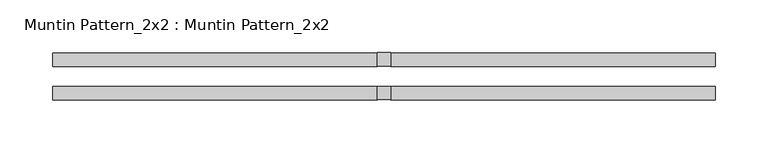
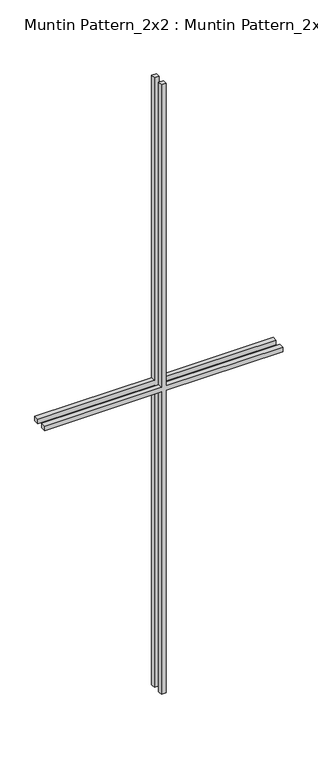
"""IFC4 building model written with IfcOpenShell, lengths in millimetres: proxy geometry, Muntin Pattern_2x2 : Muntin Pattern_2x2."""

from ifc_helpers import new_model, si_unit, frame, origin, place, context, project, spatial, polyline, outline, extrude, source, transform, mapped, element, save


def muntin_pattern_2x2_muntin_pattern_2x2_09b00a1c(model_context):
    return source(origin(), model_context, "Body", "SweptSolid", [
        extrude(outline(polyline([(850.9, -6.35), (850.9, -312.7375), (838.2, -312.7375), (838.2, -6.35), (0.0, -6.35), (0.0, 6.35), (838.2, 6.35), (838.2, 312.7375), (850.9, 312.7375), (850.9, 6.35), (1689.1, 6.35), (1689.1, -6.35), (850.9, -6.35)])), frame((0.0, -22.225, 0.0), z_axis=(0.0, 1.0, 0.0), x_axis=(0.0, 0.0, 1.0)), (0.0, 0.0, 1.0), 12.7),
        extrude(outline(polyline([(850.9, -6.35), (850.9, -312.7375), (838.2, -312.7375), (838.2, -6.35), (0.0, -6.35), (0.0, 6.35), (838.2, 6.35), (838.2, 312.7375), (850.9, 312.7375), (850.9, 6.35), (1689.1, 6.35), (1689.1, -6.35), (850.9, -6.35)])), frame((0.0, 9.525, 0.0), z_axis=(0.0, 1.0, 0.0), x_axis=(0.0, 0.0, 1.0)), (0.0, 0.0, 1.0), 12.7),
    ])


if __name__ == "__main__":
    model = new_model("IFC4")
    model_context = context("Model", 3, world=origin())
    ifc_project = project(units=[si_unit("LENGTHUNIT", "METRE", prefix="MILLI")], contexts=[model_context])
    site = spatial("IfcSite", under=ifc_project)
    building = spatial("IfcBuilding", under=site)
    placement = place(None, origin())
    muntin_pattern_2x2_muntin_pattern_2x2_shape = muntin_pattern_2x2_muntin_pattern_2x2_09b00a1c(model_context)
    element("IfcBuildingElementProxy", 1, Name="Muntin Pattern_2x2 : Muntin Pattern_2x2", ObjectType="Muntin Pattern_2x2 : Muntin Pattern_2x2", at=placement, inside=building, context=model_context, shape_type="MappedRepresentation", body=[
        mapped(muntin_pattern_2x2_muntin_pattern_2x2_shape, transform((0.0, 0.0, 0.0), x_axis=(1.0, 0.0, 0.0), y_axis=(0.0, 1.0, 0.0), z_axis=(0.0, 0.0, 1.0))),
    ])
    save(model, "model.ifc")

# Revit data of these elements
# Type "Muntin Pattern_2x2 : Muntin Pattern_2x2"
#   Width [instance default] = 4' - 0"
#   Thickness = 0' - 0 1/2"
#   Height [instance default] = 4' - 0"
#   Distance = 0' - 0 3/4"
#   Interior Material [instance default] = none
#   Exterior Material [instance default] = none
#   Default Elevation = 0
# Element 1 (IfcBuildingElementProxy, "Muntin Pattern_2x2 : Muntin Pattern_2x2")
#   Width = 2' - 0 5/8"
#   Height = 5' - 6 1/2"
#   Interior Material = Wood - Stained
#   Exterior Material = Clad - White
#   Materials on its faces: "Clad - White", "Wood - Stained"
# Materials
#   "Clad - White": class "Wood", colour RGB 242 242 238, transparency 0, Cost = 0
#   "Wood - Stained": class "Wood", colour RGB 224 178 126, transparency 0, Cost = 0
